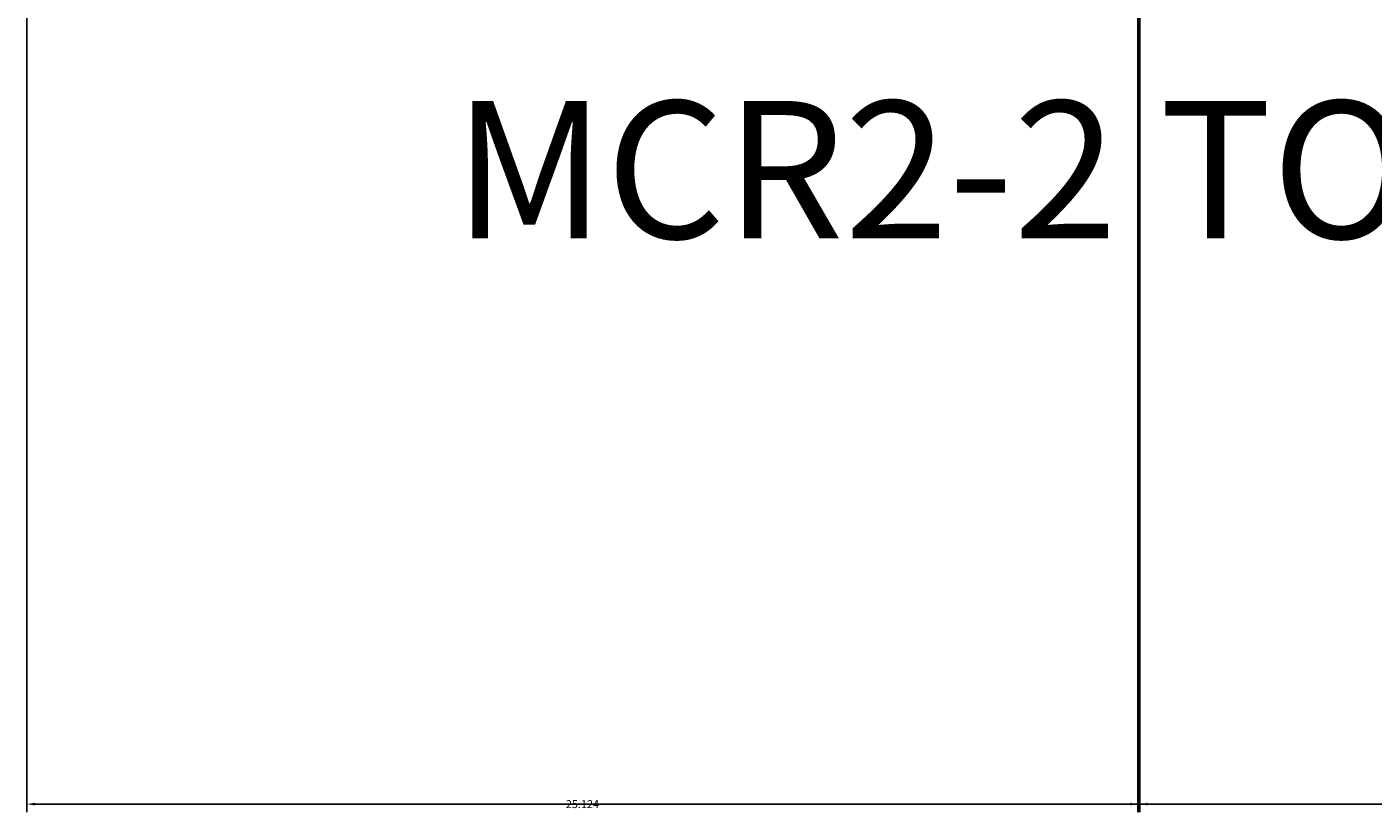
# Model space of a CAD drawing. Units: inches. Extents: x 738 to 1068, y 378 to 757.
# Tile 2 of 41: x 756 to 787, y 378 to 396. Entities that reach past the tile are written whole.
import ezdxf

# ---------------------------------------------------------------- set-up
doc = ezdxf.new("R2010")
doc.units = ezdxf.units.IN
doc.header["$MEASUREMENT"] = 0
doc.layers.add('A-ANNO-DIMS', color=2, linetype='Continuous', lineweight=18)
doc.layers.add('E-ANNO-TEXT', color=7, linetype='Continuous', lineweight=18)
doc.styles.get("Standard").update_dxf_attribs({"font": 'arial.ttf'})
doc.dimstyles.get("Standard").update_dxf_attribs({"dimtxt": 0.18, "dimasz": 0.18, "dimexe": 0.18, "dimexo": 0.0625, "dimgap": 0.09, "dimtad": 0, "dimtih": 1, "dimtoh": 1, "dimdec": 4, "dimzin": 0, "dimdsep": 46, "dimtxsty": 'Standard', "dimcen": 0.09, "dimadec": 0, "dimazin": 0, "dimtfac": 1, "dimtdec": 4, "dimtofl": 0, "dimtmove": 0, "dimatfit": 3, "dimfxl": 1, "dimtolj": 1, "dimtzin": 0, "dimarcsym": 0})

# ---------------------------------------------------------------- blocks, each defined once
blk = doc.blocks.new('*D17')
at = {"layer": 'A-ANNO-DIMS', "color": 0, "lineweight": -2, "transparency": 16777216}
for p, q in [((756.324, 415.842), (756.324, 378.239)), ((1050.049, 415.919), (1050.049, 378.239)), ((756.504, 378.419), (902.791, 378.419)), ((1049.869, 378.419), (903.582, 378.419))]:
    blk.add_line(p, q, dxfattribs=at)
at = {"layer": 'A-ANNO-DIMS', "color": 0, "transparency": 16777216}
for points in [[(756.504, 378.449), (756.504, 378.389), (756.324, 378.419)], [(1049.869, 378.449), (1049.869, 378.389), (1050.049, 378.419)]]:
    blk.add_solid(points, dxfattribs=at)
at = {"layer": 'Defpoints', "color": 0, "transparency": 16777216}
for p in [(756.324, 415.904), (1050.049, 415.982), (1050.049, 378.419)]:
    blk.add_point(p, dxfattribs=at)
at = {"layer": 'A-ANNO-DIMS', "color": 0, "transparency": 16777216, "insert": (903.186, 378.419), "char_height": 0.18, "attachment_point": 5}
blk.add_mtext('\\A1;293.7', dxfattribs=at)
blk = doc.blocks.new('*D25')
at = {"layer": 'A-ANNO-DIMS', "color": 0, "lineweight": -2, "transparency": 16777216}
for p, q in [((781.49, 646.923), (781.49, 378.239)), ((803.522, 646.923), (803.522, 378.239)), ((781.67, 378.419), (792.111, 378.419)), ((803.342, 378.419), (792.901, 378.419))]:
    blk.add_line(p, q, dxfattribs=at)
at = {"layer": 'A-ANNO-DIMS', "color": 0, "transparency": 16777216}
for points in [[(781.67, 378.449), (781.67, 378.389), (781.49, 378.419)], [(803.342, 378.449), (803.342, 378.389), (803.522, 378.419)]]:
    blk.add_solid(points, dxfattribs=at)
at = {"layer": 'Defpoints', "color": 0, "transparency": 16777216}
for p in [(781.49, 646.985), (803.522, 646.985), (803.522, 378.419)]:
    blk.add_point(p, dxfattribs=at)
at = {"layer": 'A-ANNO-DIMS', "color": 0, "transparency": 16777216, "insert": (792.506, 378.419), "char_height": 0.18, "attachment_point": 5}
blk.add_mtext('\\A1;22.03', dxfattribs=at)
blk = doc.blocks.new('*D34')
at = {"layer": 'A-ANNO-DIMS', "color": 0, "lineweight": -2, "transparency": 16777216}
for p, q in [((781.49, 686.266), (781.49, 378.239)), ((830.489, 686.266), (830.489, 378.239)), ((781.67, 378.419), (805.767, 378.419)), ((830.309, 378.419), (806.212, 378.419))]:
    blk.add_line(p, q, dxfattribs=at)
at = {"layer": 'A-ANNO-DIMS', "color": 0, "transparency": 16777216}
for points in [[(781.67, 378.449), (781.67, 378.389), (781.49, 378.419)], [(830.309, 378.449), (830.309, 378.389), (830.489, 378.419)]]:
    blk.add_solid(points, dxfattribs=at)
at = {"layer": 'Defpoints', "color": 0, "transparency": 16777216}
for p in [(781.49, 686.329), (830.489, 686.329), (830.489, 378.419)]:
    blk.add_point(p, dxfattribs=at)
at = {"layer": 'A-ANNO-DIMS', "color": 0, "transparency": 16777216, "insert": (805.99, 378.419), "char_height": 0.18, "attachment_point": 5}
blk.add_mtext('\\A1;49', dxfattribs=at)
blk = doc.blocks.new('*D38')
at = {"layer": 'A-ANNO-DIMS', "color": 0, "lineweight": -2, "transparency": 16777216}
for p, q in [((781.485, 593.017), (781.485, 378.239)), ((887.04, 593.067), (887.04, 378.239)), ((781.665, 378.419), (833.807, 378.419)), ((886.86, 378.419), (834.718, 378.419))]:
    blk.add_line(p, q, dxfattribs=at)
at = {"layer": 'A-ANNO-DIMS', "color": 0, "transparency": 16777216}
for points in [[(781.665, 378.449), (781.665, 378.389), (781.485, 378.419)], [(886.86, 378.449), (886.86, 378.389), (887.04, 378.419)]]:
    blk.add_solid(points, dxfattribs=at)
at = {"layer": 'Defpoints', "color": 0, "transparency": 16777216}
for p in [(781.485, 593.08), (887.04, 593.13), (887.04, 378.419)]:
    blk.add_point(p, dxfattribs=at)
at = {"layer": 'A-ANNO-DIMS', "color": 0, "transparency": 16777216, "insert": (834.263, 378.419), "char_height": 0.18, "attachment_point": 5}
blk.add_mtext('\\A1;105.56', dxfattribs=at)
blk = doc.blocks.new('*D40')
at = {"layer": 'A-ANNO-DIMS', "color": 0, "lineweight": -2, "transparency": 16777216}
for p, q in [((756.324, 415.842), (756.324, 378.239)), ((781.447, 396.307), (781.447, 378.239)), ((756.504, 378.419), (768.421, 378.419)), ((781.267, 378.419), (769.35, 378.419))]:
    blk.add_line(p, q, dxfattribs=at)
at = {"layer": 'A-ANNO-DIMS', "color": 0, "transparency": 16777216}
for points in [[(756.504, 378.449), (756.504, 378.389), (756.324, 378.419)], [(781.267, 378.449), (781.267, 378.389), (781.447, 378.419)]]:
    blk.add_solid(points, dxfattribs=at)
at = {"layer": 'Defpoints', "color": 0, "transparency": 16777216}
for p in [(756.324, 415.904), (781.447, 396.369), (781.447, 378.419)]:
    blk.add_point(p, dxfattribs=at)
at = {"layer": 'A-ANNO-DIMS', "color": 0, "transparency": 16777216, "insert": (768.885, 378.419), "char_height": 0.18, "attachment_point": 5}
blk.add_mtext('\\A1;25.124', dxfattribs=at)

msp = doc.modelspace()

# ---------------------------------------------------------------- texts
at = {"layer": 'E-ANNO-TEXT'}
msp.add_text('MCR2-2 TO OUTPUTS', height=3.107428, dxfattribs=at).set_placement((765.9672, 391.2068))

# ---------------------------------------------------------------- dimensions: what is measured, and where the dimension line sits
at = {"layer": 'A-ANNO-DIMS'}
for base, p1, p2, override, picture, middle in [((830.4893, 378.4191), (781.4897, 686.329), (830.4893, 686.329), {"dimdec": 0, "dimlfac": 1, "dimrnd": 0, "dimzin": 0, "dimdsep": 46, "dimlunit": 2}, '*D34', (805.9895, 378.4191)), ((803.5218, 378.4191), (781.4897, 646.9853), (803.5218, 646.9853), {"dimdec": 2, "dimlfac": 1, "dimrnd": 0, "dimzin": 0, "dimdsep": 46, "dimlunit": 2}, '*D25', (792.5057, 378.4191)), ((887.0404, 378.4191), (781.4846, 593.0796), (887.0404, 593.1296), {"dimdec": 2, "dimlfac": 1, "dimrnd": 0, "dimzin": 0, "dimdsep": 46, "dimlunit": 2}, '*D38', (834.2625, 378.4191)), ((1050.0492, 378.4191), (756.3236, 415.904), (1050.0492, 415.982), {"dimdec": 1, "dimlfac": 1, "dimrnd": 0, "dimzin": 0, "dimdsep": 46, "dimlunit": 2}, '*D17', (903.1864, 378.4191)), ((781.4474, 378.4191), (756.3236, 415.904), (781.4474, 396.3691), {"dimdec": 3, "dimlfac": 1, "dimrnd": 0, "dimzin": 0, "dimdsep": 46, "dimlunit": 2}, '*D40', (768.8855, 378.4191))]:
    dim = msp.add_linear_dim(base=base, p1=p1, p2=p2, dimstyle='Standard', override=override, dxfattribs=at)
    dim.commit()
    dim.dimension.update_dxf_attribs({"geometry": picture, "text_midpoint": middle})

doc.saveas('drawing.dxf')
